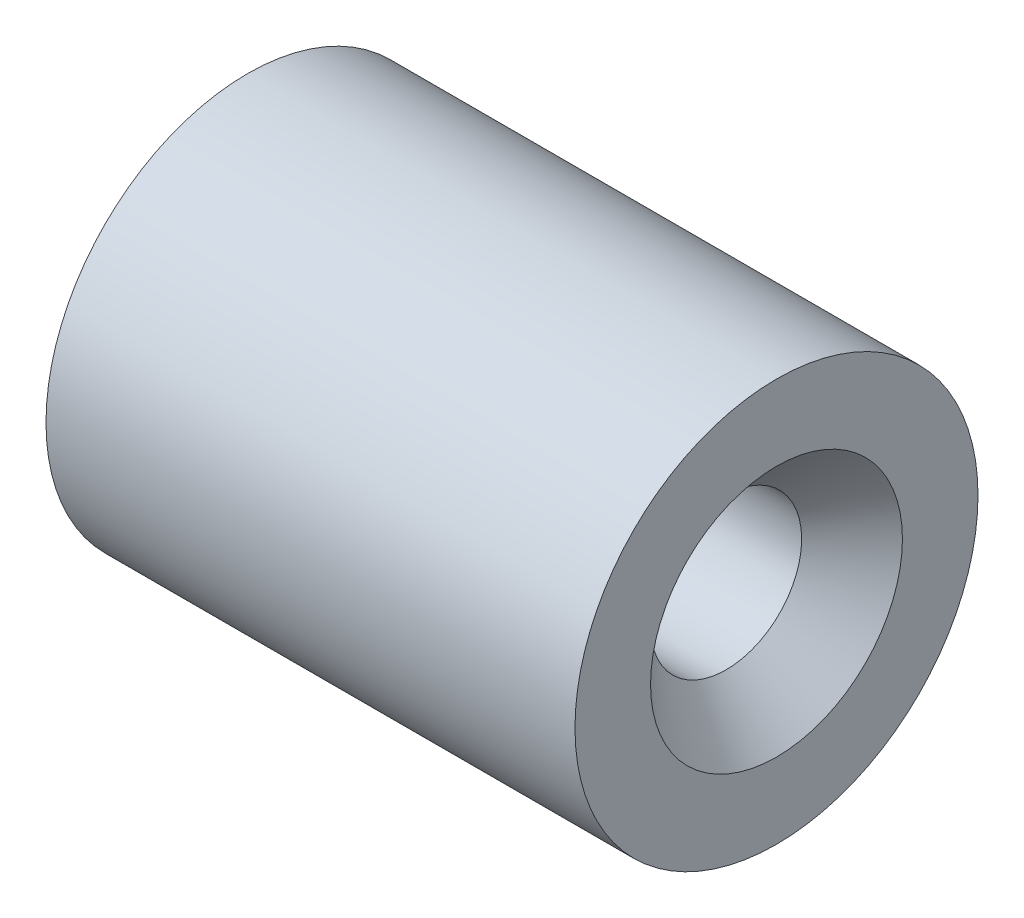
from build123d import *


with BuildPart() as part:
    # Bush Profile Sketch → Bush Body (revolve)
    with BuildSketch(Plane.XY, mode=Mode.PRIVATE) as bush_body_sk:
        Polygon((0, 10), (-4, 6), (-38, 6), (-42, 10), (-42, 16), (0, 16), align=None)
    revolve(bush_body_sk.sketch.rotate(Axis((0, 0, 0), (-1, 0, 0)), 90), axis=Axis((0, 0, 0), (-1, 0, 0)))

    # Internal Cut Profile Sketch → Internal Revolved Cut (revolve, cut)
    with BuildSketch(Plane.XY, mode=Mode.PRIVATE) as internal_revolved_cut_sk:
        Polygon((-26.196152423, -16), (-21, -13), (-21, -16), align=None)
    revolve(internal_revolved_cut_sk.sketch.rotate(Axis((-21, 0, 0), (0, -1, 0)), 180), axis=Axis((-21, 0, 0), (0, -1, 0)), mode=Mode.SUBTRACT)


solid = part.part
